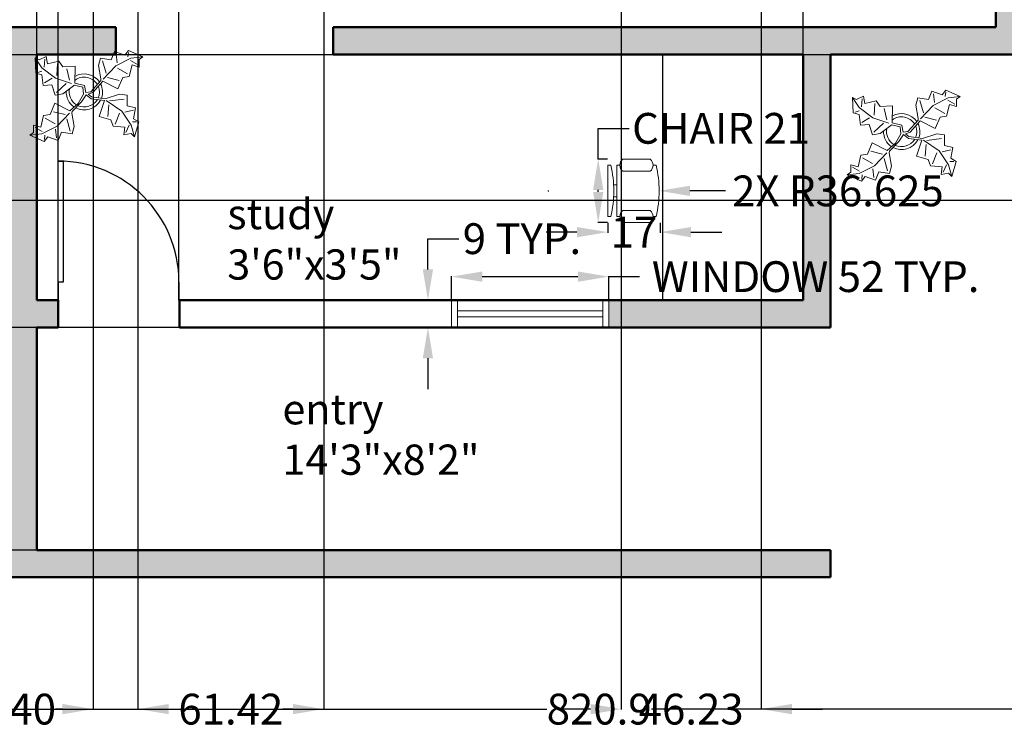
# Model space of a CAD drawing. Units: inches. Extents: x 12496 to 13538, y 6171 to 6892.
# Tile 3 of 6: x 12841 to 13167, y 6171 to 6405. Entities that reach past the tile are written whole.
import ezdxf

# ---------------------------------------------------------------- set-up
doc = ezdxf.new("R2010")
doc.units = ezdxf.units.IN
doc.header["$MEASUREMENT"] = 0
for name, color, linetype, lineweight in [('A-ANNO-DIMS', 2, 'Continuous', 18), ('A-AREA-IDEN', 7, 'Continuous', 25), ('A-DOOR', 3, 'Continuous', 25), ('A-FLOR-CASE', 8, 'Continuous', 25), ('A-FURN', 8, 'Continuous', 18), ('A-GLAZ', 4, 'Continuous', 18), ('A-WALL', 7, 'Continuous', 50), ('L-PLNT', 3, 'Continuous', 18)]:
    doc.layers.add(name, color=color, linetype=linetype, lineweight=lineweight)
doc.layers.add('A-WALL-PATT', color=18, linetype='Continuous', lineweight=13, true_color=0x000000)
doc.styles.get("Standard").update_dxf_attribs({"font": 'arial.ttf'})
doc.dimstyles.get("Standard").update_dxf_attribs({"dimtxt": 10.18, "dimasz": 10.18, "dimexe": 0.18, "dimexo": 0.0625, "dimgap": 0.09, "dimtad": 0, "dimtih": 1, "dimtoh": 1, "dimdec": 0, "dimzin": 0, "dimdsep": 46, "dimlunit": 3, "dimtxsty": 'Standard', "dimcen": 0.09, "dimadec": 0, "dimazin": 0, "dimtfac": 1, "dimtdec": 0, "dimtofl": 0, "dimtmove": 0, "dimatfit": 3, "dimfxl": 1, "dimtolj": 1, "dimtzin": 0, "dimarcsym": 0})

# ---------------------------------------------------------------- blocks, each defined once
blk = doc.blocks.new('*U2')
for p, q in [((0, 0), (0, -6)), ((40, 0), (40, -6))]:
    blk.add_line(p, q)
blk.add_lwpolyline([(0, 0), (0, 40), (1.75, 40), (1.75, 0)], close=True)
blk.add_arc((0, 0), 40, 0, 90)
blk = doc.blocks.new('Chair - Desk')
for p, q in [((-8.5, 0), (-8.5, -1)), ((-8.5, 0), (8.5, 0)), ((8.5, 0), (8.5, -1)), ((-8.5, -3), (-8.5, -4)), ((-8.5, -3), (8.5, -3)), ((-2, -3), (-2, -1.9355)), ((2, -1.9576), (2, -3)), ((8.5, -3), (8.5, -4)), ((-10.5, -5), (-10.5, -14)), ((-6.5, -14), (-6.5, -5)), ((6.5, -5), (6.5, -14)), ((10.5, -14), (10.5, -5)), ((-8.5, -15), (-8.5, -16)), ((8.5, -15), (8.5, -16))]:
    blk.add_line(p, q)
for centre, radius, start, end in [((0, 34.625), 36.625, 256.5803, 283.4197), ((-8.5, -6.5), 2.5, 36.8699, 143.1301), ((8.5, -6.5), 2.5, 36.8699, 143.1301), ((-8.5, -12.5), 2.5, 216.8699, 323.1301), ((0, 19.625), 36.625, 256.5803, 283.4197), ((8.5, -12.5), 2.5, 216.8699, 323.1301)]:
    blk.add_arc(centre, radius, start, end)
blk = doc.blocks.new('Plant - Rubber or Philodendron')
for p, q in [((8.8871, 10.7908), (9.9809, 13.4933)), ((9.9809, 13.4933), (13.3837, 12.301)), ((13.3837, 12.301), (14.68, 13.9039)), ((14.5816, 13.2037), (14.3848, 11.8033)), ((14.68, 13.9039), (19.3848, 11.8146)), ((-16.2005, 11.4774), (-13.9899, 8.1064)), ((-16.2005, 11.4774), (-14.8639, 10.7964)), ((-16.0159, 6.3329), (-16.2005, 11.4774)), ((-14.8639, 10.7964), (-12.6195, 11.8975)), ((-13.3174, 8.325), (-13.0735, 11.0065)), ((-12.6195, 11.8975), (-12.1909, 9.4345)), ((-12.1909, 9.4345), (-8.3829, 10.3)), ((-8.3829, 10.3), (-7.0549, 8.501)), ((4.6914, 8.8812), (5.3859, 11.2828)), ((5.3859, 11.2828), (8.8871, 10.7908)), ((5.9878, 10.4842), (7.1971, 6.3869)), ((15.3859, 11.3055), (10.3916, 8.7942)), ((10.5828, 12.6946), (10.8893, 9.7953)), ((15.2875, 10.6053), (17.5907, 9.2105)), ((19.3848, 11.8146), (15.3859, 11.3055)), ((19.3848, 11.8146), (18.1868, 10.9119)), ((18.1868, 10.9119), (18.1925, 8.4119)), ((-15.3434, 6.5514), (-13.9984, 6.9884)), ((-13.9899, 8.1064), (-9.5434, 4.7185)), ((-8.8369, 9.409), (-9.0894, 5.6095)), ((-7.0549, 8.501), (-3.0284, 8.6941)), ((-4.8529, 4.012), (-5.7184, 7.82)), ((-3.0284, 8.6941), (-3.0709, 3.1041)), ((4.6914, 8.8812), (5.5014, 4.4831)), ((10.3916, 8.7942), (6.2847, 4.4028)), ((14.2977, 6.1031), (10.9934, 7.9956)), ((15.7909, 9.1065), (14.8995, 5.3044)), ((18.1925, 8.4119), (15.7909, 9.1065)), ((-14.0069, 5.8704), (-16.0159, 6.3329)), ((-13.5868, 2.2894), (-14.0069, 5.8704)), ((-13.1329, 3.1804), (-10.6614, 4.727)), ((-9.5434, 4.7185), (-4.1917, 2.9888)), ((2.1141, 0.2298), (5.4346, 3.9146)), ((6.1032, 3.6844), (2.8262, -0.031)), ((5.4346, 3.9146), (5.5014, 4.4831)), ((11.1089, 1.1958), (6.1032, 3.6844)), ((7.7005, 4.8881), (11.5025, 3.9967)), ((12.7005, 4.8994), (11.1089, 1.1958)), ((14.8995, 5.3044), (12.7005, 4.8994)), ((-10.6784, 2.491), (-13.5868, 2.2894)), ((-9.5858, -0.8715), (-10.6784, 2.491)), ((-9.1318, 0.0195), (-5.9793, 2.9025)), ((-7.1228, -0.443), (-3.5248, 2.2131)), ((-3.5248, 2.2131), (-3.3011, 2.4355)), ((-3.3011, 2.4355), (-0.5306, 1.7947)), ((-3.0709, 3.1041), (0.0797, 2.3163)), ((-0.5306, 1.7947), (-0.2255, -0.5527)), ((-0.5306, 1.7947), (-0.5306, 1.7947)), ((0.0797, 2.3163), (0.4866, -0.031)), ((0.4866, -0.031), (2.1141, 0.2298)), ((-7.1228, -0.443), (-9.5858, -0.8715)), ((-4.0579, -6.2781), (-0.9375, -3.1608)), ((-2.019, -3.6148), (-0.2255, -0.5527)), ((-0.9375, -3.1608), (0.5883, -0.8135)), ((0.5883, -0.8135), (2.2447, -2.0916)), ((2.8262, -0.031), (1.3003, -0.5527)), ((1.3003, -0.5527), (2.4193, -1.4655)), ((2.2447, -2.0916), (6.7108, -2.6626)), ((2.4193, -1.4655), (6.895, -2.1175)), ((4.943, -7.9659), (6.7108, -2.6626)), ((11.6605, -0.5413), (6.895, -2.1175)), ((12.3677, -6.1981), (7.219, -2.6772)), ((8.3544, -2.7453), (13.1973, -2.1704)), ((11.6605, -0.5413), (14.1354, -0.8948)), ((14.1354, -0.8948), (14.1354, -4.4304)), ((-11.3237, -7.2629), (-9.7321, -3.5593)), ((-6.3237, -7.2516), (-10.1257, -6.3602)), ((-9.7321, -3.5593), (-4.7264, -6.0479)), ((-2.019, -3.6148), (-4.7264, -6.0479)), ((-4.1246, -6.8466), (-4.0579, -6.2781)), ((8.125, -4.0768), (7.7715, -7.9659)), ((15.5496, -10.7943), (12.3677, -6.1981)), ((16.2567, -5.8446), (13.4283, -6.5517)), ((14.1354, -4.4304), (16.9638, -5.1375)), ((16.9638, -5.1375), (16.2567, -8.673)), ((-14.4141, -11.4699), (-13.5228, -7.6679)), ((-13.5228, -7.6679), (-11.3237, -7.2629)), ((-12.921, -8.4665), (-9.6166, -10.359)), ((-9.0148, -11.1577), (-4.9047, -6.8122)), ((-4.611, -12.8477), (-5.8203, -8.7504)), ((-3.3146, -11.2447), (-4.1246, -6.8466)), ((8.8321, -9.0266), (4.943, -7.9659)), ((9.5392, -11.1479), (8.8321, -9.0266)), ((10.2463, -10.4408), (11.6605, -6.9053)), ((17.3174, -9.7337), (15.9032, -9.7337)), ((16.2567, -8.673), (18.0245, -9.7337)), ((18.0245, -9.7337), (16.6103, -14.6834)), ((-16.8157, -10.7754), (-14.4141, -11.4699)), ((-16.8101, -13.2754), (-16.8157, -10.7754)), ((-13.9107, -12.9688), (-16.2139, -11.574)), ((-14.0091, -13.669), (-9.0148, -11.1577)), ((-9.206, -15.0581), (-9.5126, -12.1588)), ((-3.3146, -11.2447), (-4.0092, -13.6463)), ((13.4283, -11.5015), (9.5392, -11.1479)), ((13.0748, -13.9763), (13.4283, -11.5015)), ((14.8425, -10.7943), (13.7819, -13.2692)), ((16.6103, -14.6834), (15.5496, -10.7943)), ((-18.008, -14.1781), (-16.8101, -13.2754)), ((-18.008, -14.1781), (-14.0091, -13.669)), ((-13.3032, -16.2674), (-18.008, -14.1781)), ((-12.0069, -14.6645), (-13.3032, -16.2674)), ((-13.2048, -15.5672), (-13.008, -14.1668)), ((-8.6042, -15.8568), (-12.0069, -14.6645)), ((-7.5103, -13.1543), (-8.6042, -15.8568)), ((-4.0092, -13.6463), (-7.5103, -13.1543)), ((15.5496, -13.6228), (13.0748, -13.9763)), ((16.6103, -14.6834), (15.5496, -13.6228))]:
    blk.add_line(p, q)
for centre, radius, start, end in [((0, 0), 6.1275, 34.37569, 120.1028), ((-0.0601, -0.2075), 5.2461, 33.82192, 124.9414), ((0.0308, 0.1664), 6, 178.6147, 235.1169), ((0.0308, 0.1664), 5, 168.1647, 238.6725), ((-0.2664, 0.1682), 5.2775, 338.4094, 20.03007), ((-0.098, 0.1364), 6.1288, 341.2017, 26.09184), ((-0.0234, 0.3825), 6.1492, 242.5812, 331.2714), ((-0.1102, 0.4886), 5.2883, 247.3711, 327.472)]:
    blk.add_arc(centre, radius, start, end)
blk = doc.blocks.new('WIN-48IN')
for p, q in [((0, 0), (0, 9)), ((2, 0), (2, 9)), ((50, 0), (50, 9)), ((52, 0), (52, 9)), ((2, 5.5), (50, 5.5)), ((2, 3.5), (50, 3.5))]:
    blk.add_line(p, q)
blk = doc.blocks.new('*D31')
at = {"layer": 'A-ANNO-DIMS', "color": 0, "lineweight": -2, "transparency": 16777216}
for p, q in [((12983.77, 6312.58), (12983.77, 6320.5)), ((12993.95, 6320.32), (13025.59, 6320.32)), ((13035.77, 6312.58), (13035.77, 6320.5)), ((13035.77, 6320.32), (13045.95, 6320.32))]:
    blk.add_line(p, q, dxfattribs=at)
at = {"layer": 'A-ANNO-DIMS', "color": 0, "transparency": 16777216}
for points in [[(12993.95, 6322.02), (12993.95, 6318.63), (12983.77, 6320.32)], [(13025.59, 6322.02), (13025.59, 6318.63), (13035.77, 6320.32)]]:
    blk.add_solid(points, dxfattribs=at)
at = {"layer": 'Defpoints', "color": 0, "transparency": 16777216}
for p in [(13035.77, 6320.32), (12983.77, 6312.52), (13035.77, 6312.52)]:
    blk.add_point(p, dxfattribs=at)
at = {"layer": 'A-ANNO-DIMS', "color": 0, "transparency": 16777216, "insert": (13104.2, 6320.32), "char_height": 10.18, "attachment_point": 5}
blk.add_mtext('\\A1;WINDOW 52 TYP.', dxfattribs=at)
blk = doc.blocks.new('*D32')
at = {"layer": 'A-ANNO-DIMS', "color": 0, "lineweight": -2, "transparency": 16777216}
for p, q in [((12975.97, 6322.7), (12975.97, 6332.88)), ((12975.97, 6332.88), (12986.15, 6332.88)), ((12983.71, 6312.52), (12975.79, 6312.52)), ((12983.71, 6303.52), (12975.79, 6303.52)), ((12975.97, 6293.34), (12975.97, 6283.16))]:
    blk.add_line(p, q, dxfattribs=at)
at = {"layer": 'A-ANNO-DIMS', "color": 0, "transparency": 16777216}
for points in [[(12974.27, 6322.7), (12977.66, 6322.7), (12975.97, 6312.52)], [(12974.27, 6293.34), (12977.66, 6293.34), (12975.97, 6303.52)]]:
    blk.add_solid(points, dxfattribs=at)
at = {"layer": 'Defpoints', "color": 0, "transparency": 16777216}
for p in [(12975.97, 6312.52), (12983.77, 6312.52), (12983.77, 6303.52)]:
    blk.add_point(p, dxfattribs=at)
at = {"layer": 'A-ANNO-DIMS', "color": 0, "transparency": 16777216, "insert": (13007.06, 6332.88), "char_height": 10.18, "attachment_point": 5}
blk.add_mtext('\\A1;9 TYP.', dxfattribs=at)
blk = doc.blocks.new('*D55')
at = {"layer": 'A-ANNO-DIMS', "color": 0, "lineweight": -2, "transparency": 16777216}
for p, q in [((13032.29, 6359.19), (13032.29, 6369.37)), ((13032.29, 6369.37), (13042.47, 6369.37)), ((13035.38, 6359.19), (13032.11, 6359.19)), ((13032.29, 6348.37), (13032.29, 6349.01)), ((13035.38, 6338.19), (13032.11, 6338.19))]:
    blk.add_line(p, q, dxfattribs=at)
at = {"layer": 'A-ANNO-DIMS', "color": 0, "transparency": 16777216}
for points in [[(13030.59, 6349.01), (13033.99, 6349.01), (13032.29, 6359.19)], [(13030.59, 6348.37), (13033.99, 6348.37), (13032.29, 6338.19)]]:
    blk.add_solid(points, dxfattribs=at)
at = {"layer": 'Defpoints', "color": 0, "transparency": 16777216}
for p in [(13032.29, 6359.19), (13035.44, 6359.19), (13035.44, 6338.19)]:
    blk.add_point(p, dxfattribs=at)
at = {"layer": 'A-ANNO-DIMS', "color": 0, "transparency": 16777216, "insert": (13072.91, 6369.37), "char_height": 10.18, "attachment_point": 5}
blk.add_mtext('\\A1;CHAIR 21', dxfattribs=at)
blk = doc.blocks.new('*D56')
at = {"layer": 'A-ANNO-DIMS', "color": 0, "lineweight": -2, "transparency": 16777216}
for p, q in [((13035.44, 6338.12), (13035.44, 6334.86)), ((13052.77, 6338.12), (13052.77, 6334.86)), ((13025.26, 6335.04), (13015.08, 6335.04)), ((13062.95, 6335.04), (13073.13, 6335.04))]:
    blk.add_line(p, q, dxfattribs=at)
at = {"layer": 'A-ANNO-DIMS', "color": 0, "transparency": 16777216}
for points in [[(13025.26, 6336.73), (13025.26, 6333.34), (13035.44, 6335.04)], [(13062.95, 6336.73), (13062.95, 6333.34), (13052.77, 6335.04)]]:
    blk.add_solid(points, dxfattribs=at)
at = {"layer": 'Defpoints', "color": 0, "transparency": 16777216}
for p in [(13035.44, 6338.19), (13052.77, 6338.19), (13035.44, 6335.04)]:
    blk.add_point(p, dxfattribs=at)
at = {"layer": 'A-ANNO-DIMS', "color": 0, "transparency": 16777216, "insert": (13044.11, 6335.04), "char_height": 10.18, "attachment_point": 5}
blk.add_mtext('\\A1;17', dxfattribs=at)
blk = doc.blocks.new('*D59')
at = {"layer": 'A-ANNO-DIMS', "color": 0, "lineweight": -2, "transparency": 16777216}
for p, q in [((12622.17, 6220.83), (12622.17, 6177.12)), ((13443.03, 6220.83), (13443.03, 6177.12)), ((12632.35, 6177.3), (13015.32, 6177.3)), ((13432.85, 6177.3), (13049.88, 6177.3))]:
    blk.add_line(p, q, dxfattribs=at)
at = {"layer": 'A-ANNO-DIMS', "color": 0, "transparency": 16777216}
for points in [[(12632.35, 6179), (12632.35, 6175.6), (12622.17, 6177.3)], [(13432.85, 6179), (13432.85, 6175.6), (13443.03, 6177.3)]]:
    blk.add_solid(points, dxfattribs=at)
at = {"layer": 'Defpoints', "color": 0, "transparency": 16777216}
for p in [(12622.17, 6220.89), (13443.03, 6220.89), (13443.03, 6177.3)]:
    blk.add_point(p, dxfattribs=at)
at = {"layer": 'A-ANNO-DIMS', "color": 0, "transparency": 16777216, "insert": (13032.6, 6177.3), "char_height": 10.18, "attachment_point": 5}
blk.add_mtext('\\A1;820.9', dxfattribs=at)
blk = doc.blocks.new('*D66')
at = {"layer": 'A-ANNO-DIMS', "color": 0, "lineweight": -2, "transparency": 16777216}
for p, q in [((12846.6, 6312.58), (12846.6, 6885.67)), ((12856.78, 6885.49), (12955.96, 6885.49)), ((13089.92, 6885.49), (12990.74, 6885.49)), ((13100.1, 6312.58), (13100.1, 6885.67))]:
    blk.add_line(p, q, dxfattribs=at)
at = {"layer": 'A-ANNO-DIMS', "color": 0, "transparency": 16777216}
for points in [[(12856.78, 6887.18), (12856.78, 6883.79), (12846.6, 6885.49)], [(13089.92, 6887.18), (13089.92, 6883.79), (13100.1, 6885.49)]]:
    blk.add_solid(points, dxfattribs=at)
at = {"layer": 'Defpoints', "color": 0, "transparency": 16777216}
for p in [(13100.1, 6885.49), (12846.6, 6312.52), (13100.1, 6312.52)]:
    blk.add_point(p, dxfattribs=at)
at = {"layer": 'A-ANNO-DIMS', "color": 0, "transparency": 16777216, "insert": (12973.35, 6885.49), "char_height": 10.18, "attachment_point": 5}
blk.add_mtext('\\A1;253.5', dxfattribs=at)
blk = doc.blocks.new('*D71')
at = {"layer": 'A-ANNO-DIMS', "color": 0, "lineweight": -2, "transparency": 16777216}
for p, q in [((13109.04, 6303.52), (12527.4, 6303.52)), ((12527.58, 6293.34), (12527.58, 6272)), ((12527.58, 6240.07), (12527.58, 6261.42)), ((13109.04, 6229.89), (12527.4, 6229.89))]:
    blk.add_line(p, q, dxfattribs=at)
at = {"layer": 'A-ANNO-DIMS', "color": 0, "transparency": 16777216}
for points in [[(12525.88, 6293.34), (12529.28, 6293.34), (12527.58, 6303.52)], [(12525.88, 6240.07), (12529.28, 6240.07), (12527.58, 6229.89)]]:
    blk.add_solid(points, dxfattribs=at)
at = {"layer": 'Defpoints', "color": 0, "transparency": 16777216}
for p in [(12527.58, 6303.52), (13109.1, 6303.52), (13109.1, 6229.89)]:
    blk.add_point(p, dxfattribs=at)
at = {"layer": 'A-ANNO-DIMS', "color": 0, "transparency": 16777216, "insert": (12527.58, 6266.71), "char_height": 10.18, "attachment_point": 5}
blk.add_mtext('\\A1;73.63', dxfattribs=at)
blk = doc.blocks.new('*D72')
at = {"layer": 'A-ANNO-DIMS', "color": 0, "lineweight": -2, "transparency": 16777216}
for p, q in [((12734.45, 6393.81), (13486.8, 6393.81)), ((13486.62, 6383.63), (13486.62, 6374.97)), ((13486.62, 6355.74), (13486.62, 6364.4)), ((12734.45, 6345.56), (13486.8, 6345.56))]:
    blk.add_line(p, q, dxfattribs=at)
at = {"layer": 'A-ANNO-DIMS', "color": 0, "transparency": 16777216}
for points in [[(13484.92, 6383.63), (13488.32, 6383.63), (13486.62, 6393.81)], [(13484.92, 6355.74), (13488.32, 6355.74), (13486.62, 6345.56)]]:
    blk.add_solid(points, dxfattribs=at)
at = {"layer": 'Defpoints', "color": 0, "transparency": 16777216}
for p in [(12734.39, 6393.81), (13486.62, 6393.81), (12734.39, 6345.56)]:
    blk.add_point(p, dxfattribs=at)
at = {"layer": 'A-ANNO-DIMS', "color": 0, "transparency": 16777216, "insert": (13486.62, 6369.69), "char_height": 10.18, "attachment_point": 5}
blk.add_mtext('\\A1;48.25', dxfattribs=at)
blk = doc.blocks.new('*D81')
at = {"layer": 'A-ANNO-DIMS', "color": 0, "lineweight": -2, "transparency": 16777216}
for p, q in [((12880.07, 6781.83), (12880.07, 6177.12)), ((12941.5, 6781.83), (12941.5, 6177.12)), ((12890.25, 6177.3), (12893.54, 6177.3)), ((12931.32, 6177.3), (12928.02, 6177.3))]:
    blk.add_line(p, q, dxfattribs=at)
at = {"layer": 'A-ANNO-DIMS', "color": 0, "transparency": 16777216}
for points in [[(12890.25, 6179), (12890.25, 6175.6), (12880.07, 6177.3)], [(12931.32, 6179), (12931.32, 6175.6), (12941.5, 6177.3)]]:
    blk.add_solid(points, dxfattribs=at)
at = {"layer": 'Defpoints', "color": 0, "transparency": 16777216}
for p in [(12880.07, 6781.89), (12941.5, 6781.89), (12941.5, 6177.3)]:
    blk.add_point(p, dxfattribs=at)
at = {"layer": 'A-ANNO-DIMS', "color": 0, "transparency": 16777216, "insert": (12910.78, 6177.3), "char_height": 10.18, "attachment_point": 5}
blk.add_mtext('\\A1;61.42', dxfattribs=at)
blk = doc.blocks.new('*D82')
at = {"layer": 'A-ANNO-DIMS', "color": 0, "lineweight": -2, "transparency": 16777216}
for p, q in [((13039.92, 6781.83), (13039.92, 6177.12)), ((13086.15, 6781.83), (13086.15, 6177.12)), ((13029.74, 6177.3), (13019.56, 6177.3)), ((13096.33, 6177.3), (13106.51, 6177.3))]:
    blk.add_line(p, q, dxfattribs=at)
at = {"layer": 'A-ANNO-DIMS', "color": 0, "transparency": 16777216}
for points in [[(13029.74, 6179), (13029.74, 6175.6), (13039.92, 6177.3)], [(13096.33, 6179), (13096.33, 6175.6), (13086.15, 6177.3)]]:
    blk.add_solid(points, dxfattribs=at)
at = {"layer": 'Defpoints', "color": 0, "transparency": 16777216}
for p in [(13039.92, 6781.89), (13086.15, 6781.89), (13086.15, 6177.3)]:
    blk.add_point(p, dxfattribs=at)
at = {"layer": 'A-ANNO-DIMS', "color": 0, "transparency": 16777216, "insert": (13063.03, 6177.3), "char_height": 10.18, "attachment_point": 5}
blk.add_mtext('\\A1;46.23', dxfattribs=at)
blk = doc.blocks.new('*D84')
at = {"layer": 'A-ANNO-DIMS', "color": 0, "lineweight": -2, "transparency": 16777216}
for p, q in [((12853.64, 6312.58), (12853.64, 6885.67)), ((12863.82, 6885.49), (12866.07, 6885.49)), ((12883.46, 6885.49), (12881.21, 6885.49)), ((12893.64, 6312.58), (12893.64, 6885.67))]:
    blk.add_line(p, q, dxfattribs=at)
at = {"layer": 'A-ANNO-DIMS', "color": 0, "transparency": 16777216}
for points in [[(12863.82, 6887.18), (12863.82, 6883.79), (12853.64, 6885.49)], [(12883.46, 6887.18), (12883.46, 6883.79), (12893.64, 6885.49)]]:
    blk.add_solid(points, dxfattribs=at)
at = {"layer": 'Defpoints', "color": 0, "transparency": 16777216}
for p in [(12893.64, 6885.49), (12853.64, 6312.52), (12893.64, 6312.52)]:
    blk.add_point(p, dxfattribs=at)
at = {"layer": 'A-ANNO-DIMS', "color": 0, "transparency": 16777216, "insert": (12873.64, 6885.49), "char_height": 10.18, "attachment_point": 5}
blk.add_mtext('\\A1;40', dxfattribs=at)
blk = doc.blocks.new('*D87')
at = {"layer": 'A-ANNO-DIMS', "color": 0, "lineweight": -2, "transparency": 16777216}
for p, q in [((12825.27, 6572.14), (12825.27, 6177.12)), ((12865.27, 6572.14), (12865.27, 6177.12)), ((12835.45, 6177.3), (12837.7, 6177.3)), ((12855.09, 6177.3), (12852.83, 6177.3))]:
    blk.add_line(p, q, dxfattribs=at)
at = {"layer": 'A-ANNO-DIMS', "color": 0, "transparency": 16777216}
for points in [[(12835.45, 6179), (12835.45, 6175.6), (12825.27, 6177.3)], [(12855.09, 6179), (12855.09, 6175.6), (12865.27, 6177.3)]]:
    blk.add_solid(points, dxfattribs=at)
at = {"layer": 'Defpoints', "color": 0, "transparency": 16777216}
for p in [(12825.27, 6572.2), (12865.27, 6572.2), (12865.27, 6177.3)]:
    blk.add_point(p, dxfattribs=at)
at = {"layer": 'A-ANNO-DIMS', "color": 0, "transparency": 16777216, "insert": (12845.27, 6177.3), "char_height": 10.18, "attachment_point": 5}
blk.add_mtext('\\A1;40', dxfattribs=at)
blk = doc.blocks.new('*D91')
at = {"layer": 'A-ANNO-DIMS', "color": 0, "lineweight": -2, "transparency": 16777216}
for p, q in [((13015.73, 6348.69), (13015.91, 6348.69)), ((13015.82, 6348.6), (13015.82, 6348.78)), ((13074.42, 6348.69), (13062.62, 6348.69))]:
    blk.add_line(p, q, dxfattribs=at)
at = {"layer": 'A-ANNO-DIMS', "color": 0, "transparency": 16777216}
blk.add_solid([(13062.62, 6350.39), (13062.62, 6346.99), (13052.44, 6348.69)], dxfattribs=at)
at = {"layer": 'Defpoints', "color": 0, "transparency": 16777216}
for p in [(13015.82, 6348.69), (13052.44, 6348.69)]:
    blk.add_point(p, dxfattribs=at)
at = {"layer": 'A-ANNO-DIMS', "color": 0, "transparency": 16777216, "insert": (13111.57, 6348.69), "char_height": 10.18, "attachment_point": 5}
blk.add_mtext('\\A1;2X R36.625', dxfattribs=at)

msp = doc.modelspace()

# ---------------------------------------------------------------- hatches: boundary and pattern name
at = {"layer": 'A-WALL-PATT'}
h = msp.add_hatch(color=256, dxfattribs=at)
h.dxf.hatch_style = 1
h.paths.add_polyline_path([(13443.0285, 6790.8943), (13327.7025, 6790.8943), (13327.7025, 6781.8943), (13434.0285, 6781.8943), (13434.0285, 6572.2028), (13169.3765, 6572.2028), (13169.3765, 6576.9323), (13160.3765, 6576.9323), (13160.3765, 6563.2028), (13163.811, 6563.2028), (13163.811, 6559.305), (13172.811, 6559.305), (13172.811, 6563.2028), (13434.0285, 6563.2028), (13434.0285, 6402.794), (13331.4198, 6402.794), (13331.4198, 6393.8103), (13434.0285, 6393.8103), (13434.0285, 6220.8943), (13443.0285, 6220.8943)])
h.paths.add_polyline_path([(13172.811, 6519.305), (13163.811, 6519.305), (13163.811, 6402.8103), (12944.6655, 6402.8103), (12944.6655, 6393.8103), (13100.0985, 6393.8103), (13100.0985, 6312.5223), (13035.7682, 6312.5223), (13035.7682, 6303.5223), (13109.0985, 6303.5223), (13109.0985, 6393.8103), (13279.4198, 6393.8103), (13279.4198, 6402.8103), (13172.811, 6402.8103)])
h.paths.add_polyline_path([(13109.0985, 6229.8943), (12846.603, 6229.8943), (12846.603, 6303.5223), (12853.6371, 6303.5223), (12853.6371, 6312.5223), (12846.603, 6312.5223), (12846.603, 6393.8103), (12872.7237, 6393.8103), (12872.7237, 6402.8103), (12846.603, 6402.8103), (12837.603, 6402.8103), (12837.603, 6229.8943), (12760.3881, 6229.8943), (12760.3881, 6220.8943), (13109.0985, 6220.8943)])
h.paths.add_polyline_path([(12708.3881, 6229.8943), (12631.1731, 6229.8943), (12631.1731, 6336.5598), (12702.8967, 6336.5598), (12702.8967, 6345.5598), (12631.1731, 6345.5598), (12631.1731, 6355.6851), (12622.1731, 6355.6851), (12622.1731, 6220.8943), (12708.3881, 6220.8943)])
h.paths.add_polyline_path([(12743.3881, 6402.8103), (12631.1731, 6402.8103), (12631.1731, 6523.6486), (12622.1731, 6523.6486), (12622.1731, 6383.6851), (12631.1731, 6383.6851), (12631.1731, 6393.8103), (12734.3881, 6393.8103), (12734.3881, 6345.5598), (12731.8151, 6345.5598), (12731.8151, 6336.5598), (12734.3881, 6336.5598), (12743.3881, 6336.5598)])
h.paths.add_polyline_path([(13039.9206, 6572.2028), (13039.9206, 6638.8628), (13048.7069, 6638.8628), (13048.7069, 6647.8628), (13039.9206, 6647.8628), (12930.9211, 6647.8628), (12930.9211, 6638.8628), (13030.9206, 6638.8628), (13030.9206, 6572.2028), (12880.0706, 6572.2028), (12880.0706, 6576.9323), (12871.0706, 6576.9323), (12871.0706, 6572.2028), (12865.2657, 6572.2028), (12865.2657, 6563.2028), (13039.9206, 6563.2028)])
h.paths.add_polyline_path([(13039.9206, 6781.8943), (13086.1485, 6781.8943), (13086.1485, 6790.8943), (12969.4956, 6790.8943), (12969.4956, 6781.8943), (13030.9206, 6781.8943), (13030.9206, 6647.8628), (13039.9206, 6647.8628)])
h.paths.add_polyline_path([(13169.3765, 6781.8943), (13275.7025, 6781.8943), (13275.7025, 6790.8943), (13114.1485, 6790.8943), (13114.1485, 6781.8943), (13160.3765, 6781.8943), (13160.3765, 6647.8628), (13088.7069, 6647.8628), (13088.7069, 6638.8628), (13160.3765, 6638.8628), (13160.3765, 6616.9323), (13169.3765, 6616.9323)])

# ---------------------------------------------------------------- linework, layer by layer
at = {"layer": 'A-FLOR-CASE'}
msp.add_line((13053.5526, 6393.8103), (13053.5526, 6312.5223), dxfattribs=at)
at = {"layer": 'A-WALL'}
for p, q in [((13163.811, 6519.305), (13163.811, 6402.8103)), ((12837.603, 6402.8103), (12846.603, 6402.8103)), ((12846.603, 6402.8103), (12872.7237, 6402.8103)), ((12944.6655, 6402.8103), (12944.6655, 6393.8103)), ((12944.6655, 6402.8103), (13163.811, 6402.8103)), ((12846.603, 6312.5223), (12846.603, 6393.8103)), ((12846.603, 6393.8103), (12872.7237, 6393.8103)), ((12944.6655, 6393.8103), (13100.0985, 6393.8103)), ((13100.0985, 6312.5223), (13100.0985, 6393.8103)), ((13109.0985, 6303.5223), (13109.0985, 6393.8103)), ((13109.0985, 6393.8103), (13434.0285, 6393.8103)), ((12846.603, 6312.5223), (12853.6371, 6312.5223)), ((12853.6371, 6312.5223), (12853.6371, 6303.5223)), ((12893.6371, 6312.5223), (13100.0985, 6312.5223)), ((12893.7685, 6312.5223), (12893.7685, 6303.5223)), ((12846.603, 6229.8943), (12846.603, 6303.5223)), ((12846.603, 6303.5223), (12853.6371, 6303.5223)), ((12893.7685, 6303.5223), (13109.0985, 6303.5223)), ((12846.603, 6229.8943), (13109.0985, 6229.8943)), ((13109.0985, 6229.8943), (13109.0985, 6220.8943)), ((12622.1731, 6220.8943), (13109.0985, 6220.8943))]:
    msp.add_line(p, q, dxfattribs=at)
msp.add_lwpolyline([(12872.7237, 6402.8103), (12872.7237, 6393.8103)], dxfattribs=at)

# ---------------------------------------------------------------- block references
at = {"layer": 'A-DOOR'}
msp.add_blockref('*U2', (12853.6371, 6318.5223), dxfattribs=at)
at = {"layer": 'A-FURN', "rotation": 90}
msp.add_blockref('Chair - Desk', (13035.4406, 6348.6873), dxfattribs=at)
at = {"layer": 'A-GLAZ'}
msp.add_blockref('WIN-48IN', (12983.7683, 6303.5219), dxfattribs=at)
at = {"layer": 'L-PLNT'}
for p in [(12862.3137, 6381.2411), (13132.628, 6368.1265)]:
    msp.add_blockref('Plant - Rubber or Philodendron', p, dxfattribs=at)

# ---------------------------------------------------------------- texts
at = {"layer": 'A-AREA-IDEN', "char_height": 10, "attachment_point": 1}
for s, insert in [('study\\P3\'6"x3\'5"', (12909.6239, 6346.0138)), ('entry\\P14\'3"x8\'2"', (12927.8589, 6281.4637))]:
    msp.add_mtext_dynamic_manual_height_columns(s, width=261.947845, gutter_width=1, heights=[0], dxfattribs=dict(at, insert=insert))

# ---------------------------------------------------------------- dimensions: what is measured, and where the dimension line sits
at = {"layer": 'A-ANNO-DIMS'}
for base, p1, p2, override, picture, middle in [((13100.0985, 6885.4873), (12846.603, 6312.5223), (13100.0985, 6312.5223), {"dimdec": 1, "dimlfac": 1, "dimrnd": 0, "dimzin": 0, "dimdsep": 46, "dimlunit": 2}, '*D66', (12973.3508, 6885.4873)), ((12893.6371, 6885.4873), (12853.6371, 6312.5223), (12893.6371, 6312.5223), {"dimdec": 0, "dimlfac": 1, "dimrnd": 0, "dimzin": 0, "dimdsep": 46, "dimlunit": 2}, '*D84', (12873.6371, 6885.4873)), ((12941.49558, 6177.30135), (12880.07062, 6781.89435), (12941.49558, 6781.89435), {"dimdec": 2, "dimlfac": 1, "dimrnd": 0, "dimzin": 0, "dimdsep": 46, "dimlunit": 2}, '*D81', (12910.7831, 6177.30135)), ((13086.1485, 6177.3013), (13039.9206, 6781.8943), (13086.1485, 6781.8943), {"dimdec": 2, "dimlfac": 1, "dimrnd": 0, "dimzin": 0, "dimdsep": 46, "dimlunit": 2}, '*D82', (13063.0345, 6177.3013)), ((12865.2657, 6177.3013), (12825.2657, 6572.2028), (12865.2657, 6572.2028), {"dimdec": 0, "dimlfac": 1, "dimrnd": 0, "dimzin": 0, "dimdsep": 46, "dimlunit": 2}, '*D87', (12845.2657, 6177.3013)), ((13443.0285, 6177.3013), (12622.1731, 6220.8943), (13443.0285, 6220.8943), {"dimdec": 1, "dimlfac": 1, "dimrnd": 0, "dimzin": 0, "dimdsep": 46, "dimlunit": 2}, '*D59', (13032.6008, 6177.3013))]:
    dim = msp.add_linear_dim(base=base, p1=p1, p2=p2, dimstyle='Standard', override=override, dxfattribs=at)
    dim.commit()
    dim.dimension.update_dxf_attribs({"geometry": picture, "text_midpoint": middle})
for base, p1, p2, angle, override, picture, middle in [((13486.6215, 6393.8103), (12734.3881, 6345.5598), (12734.3881, 6393.8103), 90, {"dimdec": 2, "dimlfac": 1, "dimrnd": 0, "dimzin": 0, "dimdsep": 46, "dimlunit": 2}, '*D72', (13486.6215, 6369.6851)), ((13035.4406, 6335.0373), (13052.7739, 6338.1873), (13035.4406, 6338.1873), 180, {"dimdec": 0, "dimlfac": 1, "dimrnd": 0, "dimzin": 0, "dimdsep": 46, "dimlunit": 2}, '*D56', (13044.1073, 6335.0373)), ((12527.5801, 6303.5223), (13109.0985, 6229.8943), (13109.0985, 6303.5223), 90, {"dimdec": 2, "dimlfac": 1, "dimrnd": 0, "dimzin": 0, "dimdsep": 46, "dimlunit": 2}, '*D71', (12527.5801, 6266.7083))]:
    dim = msp.add_linear_dim(base=base, p1=p1, p2=p2, angle=angle, dimstyle='Standard', override=override, dxfattribs=at)
    dim.commit()
    dim.dimension.update_dxf_attribs({"geometry": picture, "text_midpoint": middle})
for base, p1, p2, text, picture, middle in [((13032.2906, 6359.1873), (13035.4406, 6338.1873), (13035.4406, 6359.1873), 'CHAIR <>', '*D55', (13072.9097, 6369.3673)), ((12975.9682, 6312.5223), (12983.7682, 6303.5223), (12983.7682, 6312.5223), '<> TYP.', '*D32', (13007.0599, 6332.8823))]:
    dim = msp.add_linear_dim(base=base, p1=p1, p2=p2, angle=90, text=text, dimstyle='Standard', override={"dimdec": 0, "dimlfac": 1, "dimrnd": 0, "dimzin": 0, "dimdsep": 46, "dimlunit": 2}, dxfattribs=at)
    dim.commit()
    dim.dimension.update_dxf_attribs({"geometry": picture, "text_midpoint": middle})
dim = msp.add_radius_dim(center=(13015.8156, 6348.6873), mpoint=(13052.4406, 6348.69), text='2X <>', dimstyle='Standard', override={"dimdec": 3, "dimlfac": 1, "dimrnd": 0, "dimzin": 0, "dimdsep": 46, "dimlunit": 2}, dxfattribs=at)
dim.commit()
dim.dimension.update_dxf_attribs({"geometry": '*D91', "text_midpoint": (13074.4156, 6348.6916), "dimtype": 164})
dim = msp.add_linear_dim(base=(13035.7682, 6320.3223), p1=(12983.7682, 6312.5223), p2=(13035.7682, 6312.5223), text='WINDOW <> TYP.', dimstyle='Standard', override={"dimdec": 0, "dimlfac": 1, "dimrnd": 0, "dimzin": 0, "dimdsep": 46, "dimlunit": 2}, dxfattribs=at)
dim.commit()
dim.dimension.update_dxf_attribs({"geometry": '*D31', "text_midpoint": (13104.1982, 6320.3223)})

doc.saveas('drawing.dxf')
